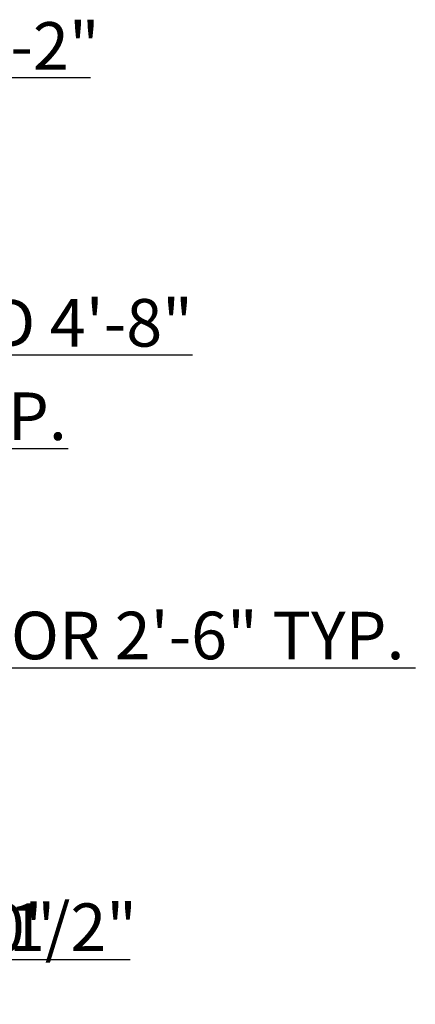
# Model space of a CAD drawing. Units: inches. Extents: x -261 to 409, y 193 to 762.
# Tile 6 of 6: x 259 to 409, y 389 to 762. Entities that reach past the tile are written whole.
import ezdxf

# ---------------------------------------------------------------- set-up
doc = ezdxf.new("R2010")
doc.units = ezdxf.units.IN
doc.layers.add('A-ANNO-DIMS', color=2, linetype='Continuous', lineweight=18)
doc.styles.get("Standard").update_dxf_attribs({"font": 'arial.ttf'})
doc.dimstyles.new('ISO-25', dxfattribs={"dimtxt": 18, "dimasz": 18, "dimexe": 1.25, "dimexo": 0.625, "dimtad": 1, "dimdec": 1, "dimlunit": 3, "dimtxsty": 'Standard', "dimcen": 2.5, "dimadec": 0, "dimazin": 0, "dimtfac": 1, "dimtdec": 1, "dimtmove": 0, "dimatfit": 3, "dimfxl": 1, "dimarcsym": 0})

# ---------------------------------------------------------------- blocks, each defined once
blk = doc.blocks.new('*D12')
at = {"layer": 'A-ANNO-DIMS', "color": 0, "lineweight": -2, "transparency": 16777216}
for p, q in [((94.3, 604.64), (94.3, 598.61)), ((130.3, 604.64), (130.3, 598.61)), ((76.3, 599.86), (58.3, 599.86)), ((94.3, 599.86), (130.3, 599.86)), ((148.3, 599.86), (277.26, 599.86))]:
    blk.add_line(p, q, dxfattribs=at)
at = {"layer": 'A-ANNO-DIMS', "color": 0, "transparency": 16777216}
for points in [[(76.3, 602.86), (76.3, 596.86), (94.3, 599.86)], [(148.3, 602.86), (148.3, 596.86), (130.3, 599.86)]]:
    blk.add_solid(points, dxfattribs=at)
at = {"layer": 'Defpoints', "color": 0, "transparency": 16777216}
for p in [(94.3, 605.26), (130.3, 605.26), (130.3, 599.86)]:
    blk.add_point(p, dxfattribs=at)
at = {"layer": 'A-ANNO-DIMS', "color": 0, "transparency": 16777216, "insert": (221.78, 609.69), "char_height": 18, "attachment_point": 5}
blk.add_mtext('3\'-0" TYP.', dxfattribs=at)
blk = doc.blocks.new('*D13')
at = {"layer": 'A-ANNO-DIMS', "color": 0, "lineweight": -2, "transparency": 16777216}
for p, q in [((150.3, 520.64), (150.3, 515.51)), ((180.3, 520.64), (180.3, 515.51)), ((132.3, 516.76), (114.3, 516.76)), ((150.3, 516.76), (180.3, 516.76)), ((198.3, 516.76), (408.8, 516.76))]:
    blk.add_line(p, q, dxfattribs=at)
at = {"layer": 'A-ANNO-DIMS', "color": 0, "transparency": 16777216}
for points in [[(132.3, 519.76), (132.3, 513.76), (150.3, 516.76)], [(198.3, 519.76), (198.3, 513.76), (180.3, 516.76)]]:
    blk.add_solid(points, dxfattribs=at)
at = {"layer": 'Defpoints', "color": 0, "transparency": 16777216}
for p in [(150.3, 521.26), (180.3, 521.26), (180.3, 516.76)]:
    blk.add_point(p, dxfattribs=at)
at = {"layer": 'A-ANNO-DIMS', "color": 0, "transparency": 16777216, "insert": (312.55, 526.7), "char_height": 18, "attachment_point": 5}
blk.add_mtext('DOOR 2\'-6" TYP.', dxfattribs=at)
blk = doc.blocks.new('*D19')
at = {"layer": 'A-ANNO-DIMS', "color": 0, "lineweight": -2, "transparency": 16777216}
for p, q in [((143.56, 642.98), (143.56, 633.98)), ((199.37, 642.98), (199.37, 633.98)), ((161.56, 635.23), (181.37, 635.23)), ((199.37, 635.23), (324.36, 635.23))]:
    blk.add_line(p, q, dxfattribs=at)
at = {"layer": 'A-ANNO-DIMS', "color": 0, "transparency": 16777216}
for points in [[(161.56, 638.23), (161.56, 632.23), (143.56, 635.23)], [(181.37, 638.23), (181.37, 632.23), (199.37, 635.23)]]:
    blk.add_solid(points, dxfattribs=at)
at = {"layer": 'Defpoints', "color": 0, "transparency": 16777216}
for p in [(143.56, 643.61), (199.37, 643.61), (199.37, 635.23)]:
    blk.add_point(p, dxfattribs=at)
at = {"layer": 'A-ANNO-DIMS', "color": 0, "transparency": 16777216, "insert": (270.87, 645.05), "char_height": 18, "attachment_point": 5}
blk.add_mtext('BED 4\'-8"', dxfattribs=at)
blk = doc.blocks.new('*D37')
at = {"layer": 'A-ANNO-DIMS', "color": 0, "lineweight": -2, "transparency": 16777216}
for p, q in [((154.3, 556.64), (154.3, 405.1)), ((202.3, 556.64), (202.3, 405.1)), ((172.3, 406.35), (184.3, 406.35)), ((202.3, 406.35), (270.13, 406.35))]:
    blk.add_line(p, q, dxfattribs=at)
at = {"layer": 'A-ANNO-DIMS', "color": 0, "transparency": 16777216}
for points in [[(172.3, 409.35), (172.3, 403.35), (154.3, 406.35)], [(184.3, 409.35), (184.3, 403.35), (202.3, 406.35)]]:
    blk.add_solid(points, dxfattribs=at)
at = {"layer": 'Defpoints', "color": 0, "transparency": 16777216}
for p in [(154.3, 557.26), (202.3, 557.26), (202.3, 406.35)]:
    blk.add_point(p, dxfattribs=at)
at = {"layer": 'A-ANNO-DIMS', "color": 0, "transparency": 16777216, "insert": (245.21, 416.17), "char_height": 18, "attachment_point": 5}
blk.add_mtext('4\'-0"', dxfattribs=at)
blk = doc.blocks.new('*D41')
at = {"layer": 'A-ANNO-DIMS', "color": 0, "lineweight": -2, "transparency": 16777216}
for p, q in [((130.3, 428.64), (130.3, 405.1)), ((177.66, 428.64), (177.66, 405.1)), ((148.3, 406.35), (159.66, 406.35)), ((177.66, 406.35), (300.67, 406.35))]:
    blk.add_line(p, q, dxfattribs=at)
at = {"layer": 'A-ANNO-DIMS', "color": 0, "transparency": 16777216}
for points in [[(148.3, 409.35), (148.3, 403.35), (130.3, 406.35)], [(159.66, 409.35), (159.66, 403.35), (177.66, 406.35)]]:
    blk.add_solid(points, dxfattribs=at)
at = {"layer": 'Defpoints', "color": 0, "transparency": 16777216}
for p in [(130.3, 429.26), (177.66, 429.26), (177.66, 406.35)]:
    blk.add_point(p, dxfattribs=at)
at = {"layer": 'A-ANNO-DIMS', "color": 0, "transparency": 16777216, "insert": (248.17, 416.29), "char_height": 18, "attachment_point": 5}
blk.add_mtext('3\'-11 1/2"', dxfattribs=at)
blk = doc.blocks.new('*D44')
at = {"layer": 'A-ANNO-DIMS', "color": 0, "lineweight": -2, "transparency": 16777216}
for p, q in [((170.32, 740.18), (152.32, 740.18)), ((188.32, 562.25), (188.32, 741.43)), ((188.32, 740.18), (202.3, 740.18)), ((202.3, 561.89), (202.3, 741.43)), ((220.3, 740.18), (285.71, 740.18))]:
    blk.add_line(p, q, dxfattribs=at)
at = {"layer": 'A-ANNO-DIMS', "color": 0, "transparency": 16777216}
for points in [[(170.32, 743.18), (170.32, 737.18), (188.32, 740.18)], [(220.3, 743.18), (220.3, 737.18), (202.3, 740.18)]]:
    blk.add_solid(points, dxfattribs=at)
at = {"layer": 'Defpoints', "color": 0, "transparency": 16777216}
for p in [(202.3, 740.18), (188.32, 561.62), (202.3, 561.26)]:
    blk.add_point(p, dxfattribs=at)
at = {"layer": 'A-ANNO-DIMS', "color": 0, "transparency": 16777216, "insert": (262.01, 749.84), "char_height": 18, "attachment_point": 5}
blk.add_mtext('1\'-2"', dxfattribs=at)

msp = doc.modelspace()

# ---------------------------------------------------------------- dimensions: what is measured, and where the dimension line sits
at = {"layer": 'A-ANNO-DIMS'}
for base, p1, p2, picture, middle in [((202.3, 740.18), (188.32, 561.62), (202.3, 561.26), '*D44', (262.01, 749.84)), ((202.3, 406.35), (154.3, 557.26), (202.3, 557.26), '*D37', (245.21, 416.17)), ((177.66, 406.35), (130.3, 429.26), (177.66, 429.26), '*D41', (248.17, 416.29))]:
    dim = msp.add_linear_dim(base=base, p1=p1, p2=p2, dimstyle='ISO-25', override={"dimdec": 1, "dimlfac": 1, "dimrnd": 0, "dimzin": 1, "dimdsep": 46, "dimlunit": 4, "dimfrac": 2}, dxfattribs=at)
    dim.commit()
    dim.dimension.update_dxf_attribs({"geometry": picture, "text_midpoint": middle})
for base, p1, p2, text, picture, middle in [((199.37, 635.23), (143.56, 643.61), (199.37, 643.61), 'BED <>', '*D19', (270.87, 645.05)), ((130.3, 599.86), (94.3, 605.26), (130.3, 605.26), '<> TYP.', '*D12', (221.78, 609.69)), ((180.3, 516.76), (150.3, 521.26), (180.3, 521.26), 'DOOR <> TYP.', '*D13', (312.55, 526.7))]:
    dim = msp.add_linear_dim(base=base, p1=p1, p2=p2, text=text, dimstyle='ISO-25', override={"dimdec": 1, "dimlfac": 1, "dimrnd": 0, "dimzin": 1, "dimdsep": 46, "dimlunit": 4, "dimfrac": 2}, dxfattribs=at)
    dim.commit()
    dim.dimension.update_dxf_attribs({"geometry": picture, "text_midpoint": middle})

doc.saveas('drawing.dxf')
